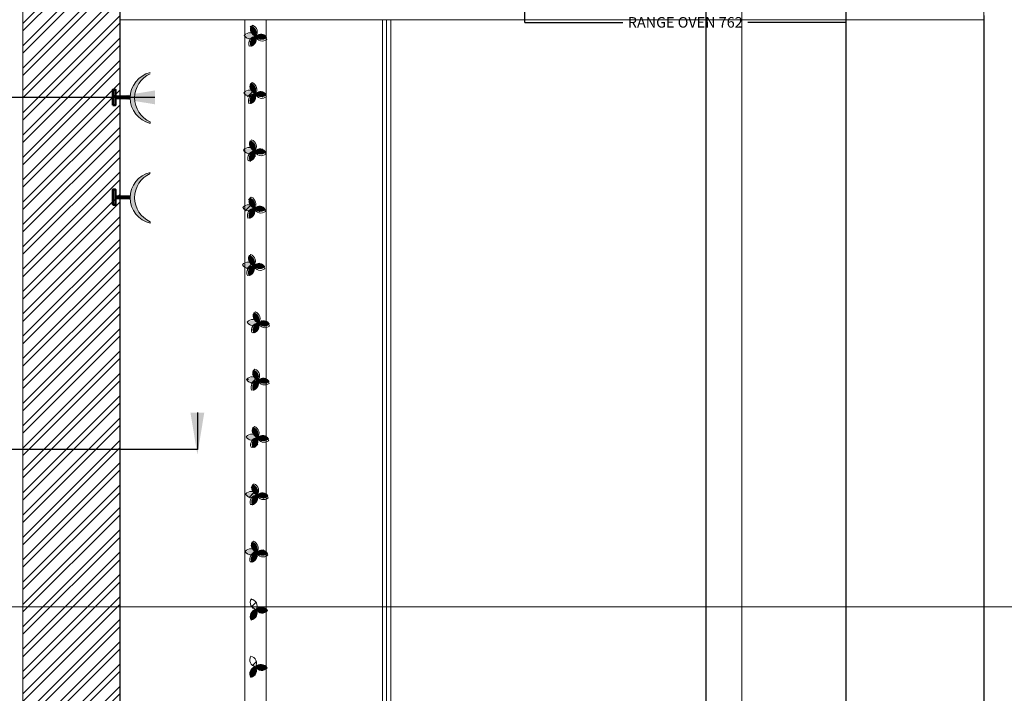
# Model space of a CAD drawing. Units: millimetres. Extents: x 1944 to 29915, y -10550 to 5909.
# Tile 7 of 24: x 6709 to 9044, y 2263 to 3861. Entities that reach past the tile are written whole.
import ezdxf
from ezdxf import colors
from ezdxf.entities.mleader import LeaderData, LeaderLine
from ezdxf.math import Vec2, Vec3

# ---------------------------------------------------------------- set-up
doc = ezdxf.new("R2010")
doc.units = ezdxf.units.MM
doc.header["$MEASUREMENT"] = 0
for name, color, linetype, lineweight in [('A-ANNO-DIMS', 2, 'Continuous', 18), ('A-ANNO-SYMB', 2, 'Continuous', 18), ('A-ANNO-TEXT', 7, 'Continuous', 25), ('A-FLOR-FIXT', 9, 'Continuous', 18), ('A-FLOR-PATT', 252, 'Continuous', 13), ('A-FURN', 8, 'Continuous', 18), ('A-WALL', 7, 'Continuous', 50), ('A-WALL-PATT', 8, 'Continuous', 18)]:
    doc.layers.add(name, color=color, linetype=linetype, lineweight=lineweight)
doc.styles.get("Standard").update_dxf_attribs({"font": 'arial.ttf'})
doc.dimstyles.get("Standard").update_dxf_attribs({"dimtxt": 25, "dimasz": 0.18, "dimexe": 0.18, "dimexo": 0.0625, "dimgap": 0.09, "dimtad": 0, "dimtih": 1, "dimtoh": 1, "dimdec": 0, "dimzin": 0, "dimdsep": 46, "dimtxsty": 'Standard', "dimcen": 0.09, "dimadec": 0, "dimazin": 0, "dimtfac": 1, "dimtdec": 0, "dimtofl": 0, "dimtmove": 0, "dimatfit": 3, "dimfxl": 1, "dimtolj": 1, "dimtzin": 0, "dimarcsym": 0})

# ---------------------------------------------------------------- blocks, each defined once
blk = doc.blocks.new('ORNAMENT-TILE')
for points in [[(27, 25, 0.520567), (15.6, 50, 0.520567)], [(27.4, 25, -0.520567), (0, 23.1, -0.520567)], [(27, 25, -0.520567), (15.6, 0, -0.520567)], [(27, 25, 0.520567), (54.3, 22.2, 0.520567)]]:
    blk.add_lwpolyline(points, format="xyb", close=True)
blk = doc.blocks.new('COAT-HOOK')
blk.add_line((47.6, 3.3), (47.6, 0))
for centre, radius, start, end in [((61.9, 60.2), 61.9, 103.3534, 256.6466), ((73.3, 60.6), 62.7, 114.1736, 245.8264)]:
    blk.add_arc(centre, radius, start, end)
blk = doc.blocks.new('*D38')
at = {"layer": 'A-ANNO-DIMS', "color": 0, "lineweight": -2, "transparency": 16777216}
for p, q in [((7906, 3968.8), (7906, 3854.4)), ((8668, 3968.8), (8668, 3854.4)), ((7906.2, 3854.5), (8138.8, 3854.5)), ((8667.9, 3854.5), (8435.3, 3854.5))]:
    blk.add_line(p, q, dxfattribs=at)
at = {"layer": 'A-ANNO-DIMS', "color": 0, "transparency": 16777216}
for points in [[(7906.2, 3854.6), (7906.2, 3854.5), (7906, 3854.5)], [(8667.9, 3854.6), (8667.9, 3854.5), (8668, 3854.5)]]:
    blk.add_solid(points, dxfattribs=at)
at = {"layer": 'Defpoints', "color": 0, "transparency": 16777216}
for p in [(7906, 3968.8), (8668, 3968.8), (8668, 3854.5)]:
    blk.add_point(p, dxfattribs=at)
at = {"layer": 'A-ANNO-DIMS', "color": 0, "transparency": 16777216, "insert": (8287, 3854.5), "char_height": 25, "attachment_point": 5}
blk.add_mtext('\\A1;RANGE OVEN 762', dxfattribs=at)
blk = doc.blocks.new('*D49')
at = {"layer": 'A-ANNO-DIMS', "color": 0, "lineweight": -2, "transparency": 16777216}
for p, q in [((8335.5, 4760.8), (8335.5, -697.2)), ((6945.9, 4530.8), (6945.9, -697.2)), ((6946.1, -697), (7589.8, -697)), ((8335.3, -697), (7691.6, -697))]:
    blk.add_line(p, q, dxfattribs=at)
at = {"layer": 'A-ANNO-DIMS', "color": 0, "transparency": 16777216}
for points in [[(6946.1, -697), (6946.1, -697.1), (6945.9, -697)], [(8335.3, -697), (8335.3, -697.1), (8335.5, -697)]]:
    blk.add_solid(points, dxfattribs=at)
at = {"layer": 'Defpoints', "color": 0, "transparency": 16777216}
for p in [(8335.5, 4760.8), (6945.9, 4530.8), (8335.5, -697)]:
    blk.add_point(p, dxfattribs=at)
at = {"layer": 'A-ANNO-DIMS', "color": 0, "transparency": 16777216, "insert": (7640.7, -697), "char_height": 25, "attachment_point": 5}
blk.add_mtext('\\A1;1389.5', dxfattribs=at)
blk = doc.blocks.new('*D57')
at = {"layer": 'A-ANNO-DIMS', "color": 0, "lineweight": -2, "transparency": 16777216}
for p, q in [((8995.2, 4760.8), (5803.8, 4760.8)), ((5804, 4760.7), (5804, 2520.7)), ((5804, 255), (5804, 2495)), ((8999.6, 254.8), (5803.8, 254.8))]:
    blk.add_line(p, q, dxfattribs=at)
at = {"layer": 'A-ANNO-DIMS', "color": 0, "transparency": 16777216}
for points in [[(5804, 4760.7), (5804, 4760.7), (5804, 4760.8)], [(5804, 255), (5804, 255), (5804, 254.8)]]:
    blk.add_solid(points, dxfattribs=at)
at = {"layer": 'Defpoints', "color": 0, "transparency": 16777216}
for p in [(8995.2, 4760.8), (5804, 254.8), (8999.6, 254.8)]:
    blk.add_point(p, dxfattribs=at)
at = {"layer": 'A-ANNO-DIMS', "color": 0, "transparency": 16777216, "insert": (5804, 2507.8), "char_height": 25, "attachment_point": 5}
blk.add_mtext('\\A1;4506', dxfattribs=at)
blk = doc.blocks.new('*D59')
at = {"layer": 'A-ANNO-DIMS', "color": 0, "lineweight": -2, "transparency": 16777216}
for p, q in [((8668, 4019.6), (8668, -697.2)), ((8995.2, 3870.8), (8995.2, -697.2)), ((8668.2, -697), (8789.5, -697)), ((8995, -697), (8873.8, -697))]:
    blk.add_line(p, q, dxfattribs=at)
at = {"layer": 'A-ANNO-DIMS', "color": 0, "transparency": 16777216}
for points in [[(8668.2, -697), (8668.2, -697.1), (8668, -697)], [(8995, -697), (8995, -697.1), (8995.2, -697)]]:
    blk.add_solid(points, dxfattribs=at)
at = {"layer": 'Defpoints', "color": 0, "transparency": 16777216}
for p in [(8668, 4019.6), (8995.2, 3870.8), (8995.2, -697)]:
    blk.add_point(p, dxfattribs=at)
at = {"layer": 'A-ANNO-DIMS', "color": 0, "transparency": 16777216, "insert": (8831.6, -697), "char_height": 25, "attachment_point": 5}
blk.add_mtext('\\A1;327.2', dxfattribs=at)

msp = doc.modelspace()

# ---------------------------------------------------------------- hatches: boundary and pattern name
at = {"layer": 'A-ANNO-SYMB'}
h = msp.add_hatch(color=256, dxfattribs=at)
h.dxf.hatch_style = 1
h.paths.add_polyline_path([(7018.308, 3614.925), (7018.308, 3618.232, -0.64725624), (7018.308, 3732.725), (7018.308, 3735.411, 0.79041326)])
h = msp.add_hatch(color=256, dxfattribs=at)
h.dxf.hatch_style = 1
h.paths.add_polyline_path([(6929.507, 3658.332), (6936.053, 3658.332), (6936.053, 3694.562), (6929.507, 3694.562)])
h = msp.add_hatch(color=256, dxfattribs=at)
h.dxf.hatch_style = 1
h.paths.add_polyline_path([(6936.053, 3678.409), (6936.053, 3674.325), (6970.696, 3674.325, -0.01650068), (6970.776, 3678.409)])
h = msp.add_hatch(color=256, dxfattribs=at)
h.dxf.hatch_style = 1
h.paths.add_polyline_path([(7018.308, 3378.048), (7018.308, 3381.355, -0.64725624), (7018.308, 3495.848), (7018.308, 3498.534, 0.79041326)])
h = msp.add_hatch(color=256, dxfattribs=at)
h.dxf.hatch_style = 1
h.paths.add_polyline_path([(6929.507, 3421.455), (6936.053, 3421.455), (6936.053, 3457.684), (6929.507, 3457.684)])
h = msp.add_hatch(color=256, dxfattribs=at)
h.dxf.hatch_style = 1
h.paths.add_polyline_path([(6936.053, 3441.532), (6936.053, 3437.447), (6970.696, 3437.447, -0.01650068), (6970.776, 3441.532)])
at = {"layer": 'A-FLOR-PATT'}
h = msp.add_hatch(color=256, dxfattribs=at)
h.dxf.hatch_style = 1
h.paths.add_polyline_path([(7256.928, 3846.567, -0.52056705), (7268.294, 3821.579, -0.52056705), (7256.928, 3796.591, -0.27363046), (7256.947, 3813.653, -0.26802551), (7241.299, 3819.656, -0.30570263), (7258.281, 3827.577, -0.31162563)])
h = msp.add_hatch(dxfattribs=at)
h.set_pattern_fill('ANSI32', color=256, scale=100)
h.paths.add_polyline_path([(7256.928, 3846.567, 0.31162563), (7258.281, 3827.577, -0.17976414), (7268.452, 3821.853, 0.51458497)])
h = msp.add_hatch(color=256, dxfattribs=at)
h.dxf.hatch_style = 1
h.paths.add_polyline_path([(7256.928, 3846.567, 0.31162563), (7258.281, 3827.577, -0.17976414), (7268.452, 3821.853, 0.51458497)])
h = msp.add_hatch(dxfattribs=at)
h.set_pattern_fill('ANSI32', color=256, scale=100)
h.paths.add_polyline_path([(7268.484, 3821.248, -0.00568537), (7268.294, 3821.579, 0.21614784), (7256.947, 3813.653, 0.21566285)], flags=16)
h.paths.add_polyline_path([(7295.606, 3818.823, -0.51336232), (7268.484, 3821.248, -0.51336232), (7256.928, 3796.591, -0.27363046), (7256.947, 3813.653, -0.26802551), (7241.299, 3819.656, -0.30570263), (7258.281, 3827.577, -0.18072738), (7268.492, 3821.805, -0.51487633)])
h.paths.add_polyline_path([(7268.484, 3821.248, -0.21566285), (7256.947, 3813.653, 0.27363046), (7256.928, 3796.591, 0.51336232)], flags=16)
h = msp.add_hatch(dxfattribs=at)
h.set_pattern_fill('ANSI32', color=256, scale=100)
h.paths.add_polyline_path([(7268.294, 3821.579, -0.17977754), (7258.281, 3827.577, 0.30570263), (7241.299, 3819.656, 0.26802551), (7256.947, 3813.653, -0.21614784)])
h.paths.add_polyline_path([(7268.484, 3821.248, -0.00568537), (7268.294, 3821.579, 0.21614784), (7256.947, 3813.653, 0.21566285)], flags=16)
h.paths.add_polyline_path([(7268.484, 3821.248, -0.21566285), (7256.947, 3813.653, 0.27363046), (7256.928, 3796.591, 0.51336232)], flags=16)
h = msp.add_hatch(color=256, dxfattribs=at)
h.dxf.hatch_style = 1
h.paths.add_polyline_path([(7256.947, 3813.653, 0.27363046), (7256.928, 3796.591, 0.51336232), (7268.484, 3821.248, -0.21566285)])
h = msp.add_hatch(color=256, dxfattribs=at)
h.dxf.hatch_style = 1
h.paths.add_polyline_path([(7268.484, 3821.248, -0.00568537), (7268.294, 3821.579, 0.21614784), (7256.947, 3813.653, 0.21566285)])
h = msp.add_hatch(color=256, dxfattribs=at)
h.dxf.hatch_style = 1
h.paths.add_polyline_path([(7258.281, 3827.577, 0.17977754), (7268.294, 3821.579, 0.00471819), (7268.452, 3821.853, 0.17976414)])
h = msp.add_hatch(color=256, dxfattribs=at)
h.dxf.hatch_style = 1
h.paths.add_polyline_path([(7268.492, 3821.805, -0.00448785), (7268.684, 3821.573, -0.00568537), (7268.484, 3821.248, 0.51336232), (7295.606, 3818.823, 0.51487633)])
h = msp.add_hatch(color=256, dxfattribs=at)
h.dxf.hatch_style = 1
h.paths.add_polyline_path([(7255.798, 3710.561, -0.52056705), (7267.164, 3685.573, -0.52056705), (7255.798, 3660.585, -0.27363046), (7255.818, 3677.648, -0.26802551), (7240.17, 3683.651, -0.30570263), (7257.151, 3691.572, -0.31162563)])
h = msp.add_hatch(dxfattribs=at)
h.set_pattern_fill('ANSI32', color=256, scale=100)
h.paths.add_polyline_path([(7267.354, 3685.243, -0.00568537), (7267.164, 3685.573, 0.21614784), (7255.818, 3677.648, 0.21566285)], flags=16)
h.paths.add_polyline_path([(7294.477, 3682.818, -0.51336232), (7267.354, 3685.243, -0.51336232), (7255.798, 3660.585, -0.27363046), (7255.818, 3677.648, -0.26802551), (7240.17, 3683.651, -0.30570263), (7257.151, 3691.572, -0.18072738), (7267.362, 3685.799, -0.51487633)])
h.paths.add_polyline_path([(7267.354, 3685.243, -0.21566285), (7255.818, 3677.648, 0.27363046), (7255.798, 3660.585, 0.51336232)], flags=16)
h = msp.add_hatch(dxfattribs=at)
h.set_pattern_fill('ANSI32', color=256, scale=100)
h.paths.add_polyline_path([(7267.164, 3685.573, -0.17977754), (7257.151, 3691.572, 0.30570263), (7240.17, 3683.651, 0.26802551), (7255.818, 3677.648, -0.21614784)])
h.paths.add_polyline_path([(7267.354, 3685.243, -0.00568537), (7267.164, 3685.573, 0.21614784), (7255.818, 3677.648, 0.21566285)], flags=16)
h.paths.add_polyline_path([(7267.354, 3685.243, -0.21566285), (7255.818, 3677.648, 0.27363046), (7255.798, 3660.585, 0.51336232)], flags=16)
h = msp.add_hatch(dxfattribs=at)
h.set_pattern_fill('ANSI32', color=256, scale=100)
h.paths.add_polyline_path([(7255.798, 3710.561, 0.31162563), (7257.151, 3691.572, -0.17976414), (7267.322, 3685.847, 0.51458497)])
h = msp.add_hatch(color=256, dxfattribs=at)
h.dxf.hatch_style = 1
h.paths.add_polyline_path([(7255.798, 3710.561, 0.31162563), (7257.151, 3691.572, -0.17976414), (7267.322, 3685.847, 0.51458497)])
h = msp.add_hatch(color=256, dxfattribs=at)
h.dxf.hatch_style = 1
h.paths.add_polyline_path([(7257.151, 3691.572, 0.17977754), (7267.164, 3685.573, 0.00471819), (7267.322, 3685.847, 0.17976414)])
h = msp.add_hatch(color=256, dxfattribs=at)
h.dxf.hatch_style = 1
h.paths.add_polyline_path([(7267.362, 3685.799, -0.00448785), (7267.554, 3685.567, -0.00568537), (7267.354, 3685.243, 0.51336232), (7294.477, 3682.818, 0.51487633)])
h = msp.add_hatch(color=256, dxfattribs=at)
h.dxf.hatch_style = 1
h.paths.add_polyline_path([(7255.818, 3677.648, 0.27363046), (7255.798, 3660.585, 0.51336232), (7267.354, 3685.243, -0.21566285)])
h = msp.add_hatch(color=256, dxfattribs=at)
h.dxf.hatch_style = 1
h.paths.add_polyline_path([(7267.354, 3685.243, -0.00568537), (7267.164, 3685.573, 0.21614784), (7255.818, 3677.648, 0.21566285)])
h = msp.add_hatch(color=256, dxfattribs=at)
h.dxf.hatch_style = 1
h.paths.add_polyline_path([(7254.668, 3574.556, -0.52056705), (7266.034, 3549.568, -0.52056705), (7254.668, 3524.58, -0.27363046), (7254.688, 3541.642, -0.26802551), (7239.04, 3547.645, -0.30570263), (7256.021, 3555.566, -0.31162563)])
h = msp.add_hatch(dxfattribs=at)
h.set_pattern_fill('ANSI32', color=256, scale=100)
h.paths.add_polyline_path([(7254.668, 3574.556, 0.31162563), (7256.021, 3555.566, -0.17976414), (7266.192, 3549.842, 0.51458497)])
h = msp.add_hatch(color=256, dxfattribs=at)
h.dxf.hatch_style = 1
h.paths.add_polyline_path([(7254.668, 3574.556, 0.31162563), (7256.021, 3555.566, -0.17976414), (7266.192, 3549.842, 0.51458497)])
h = msp.add_hatch(dxfattribs=at)
h.set_pattern_fill('ANSI32', color=256, scale=100)
h.paths.add_polyline_path([(7266.224, 3549.238, -0.00568537), (7266.034, 3549.568, 0.21614784), (7254.688, 3541.642, 0.21566285)], flags=16)
h.paths.add_polyline_path([(7293.347, 3546.812, -0.51336232), (7266.224, 3549.238, -0.51336232), (7254.668, 3524.58, -0.27363046), (7254.688, 3541.642, -0.26802551), (7239.04, 3547.645, -0.30570263), (7256.021, 3555.566, -0.18072738), (7266.233, 3549.794, -0.51487633)])
h.paths.add_polyline_path([(7266.224, 3549.238, -0.21566285), (7254.688, 3541.642, 0.27363046), (7254.668, 3524.58, 0.51336232)], flags=16)
h = msp.add_hatch(dxfattribs=at)
h.set_pattern_fill('ANSI32', color=256, scale=100)
h.paths.add_polyline_path([(7266.034, 3549.568, -0.17977754), (7256.021, 3555.566, 0.30570263), (7239.04, 3547.645, 0.26802551), (7254.688, 3541.642, -0.21614784)])
h.paths.add_polyline_path([(7266.224, 3549.238, -0.00568537), (7266.034, 3549.568, 0.21614784), (7254.688, 3541.642, 0.21566285)], flags=16)
h.paths.add_polyline_path([(7266.224, 3549.238, -0.21566285), (7254.688, 3541.642, 0.27363046), (7254.668, 3524.58, 0.51336232)], flags=16)
h = msp.add_hatch(color=256, dxfattribs=at)
h.dxf.hatch_style = 1
h.paths.add_polyline_path([(7254.688, 3541.642, 0.27363046), (7254.668, 3524.58, 0.51336232), (7266.224, 3549.238, -0.21566285)])
h = msp.add_hatch(color=256, dxfattribs=at)
h.dxf.hatch_style = 1
h.paths.add_polyline_path([(7266.224, 3549.238, -0.00568537), (7266.034, 3549.568, 0.21614784), (7254.688, 3541.642, 0.21566285)])
h = msp.add_hatch(color=256, dxfattribs=at)
h.dxf.hatch_style = 1
h.paths.add_polyline_path([(7256.021, 3555.566, 0.17977754), (7266.034, 3549.568, 0.00471819), (7266.192, 3549.842, 0.17976414)])
h = msp.add_hatch(color=256, dxfattribs=at)
h.dxf.hatch_style = 1
h.paths.add_polyline_path([(7266.233, 3549.794, -0.00448785), (7266.424, 3549.562, -0.00568537), (7266.224, 3549.238, 0.51336232), (7293.347, 3546.812, 0.51487633)])
h = msp.add_hatch(color=256, dxfattribs=at)
h.dxf.hatch_style = 1
h.paths.add_polyline_path([(7253.539, 3438.55, -0.52056705), (7264.904, 3413.563, -0.52056705), (7253.539, 3388.575, -0.27363046), (7253.558, 3405.637, -0.26802551), (7237.91, 3411.64, -0.30570263), (7254.892, 3419.561, -0.31162563)])
h = msp.add_hatch(dxfattribs=at)
h.set_pattern_fill('ANSI32', color=256, scale=100)
h.paths.add_polyline_path([(7253.539, 3438.55, 0.31162563), (7254.892, 3419.561, -0.17976414), (7265.063, 3413.836, 0.51458497)])
h = msp.add_hatch(color=256, dxfattribs=at)
h.dxf.hatch_style = 1
h.paths.add_polyline_path([(7253.539, 3438.55, 0.31162563), (7254.892, 3419.561, -0.17976414), (7265.063, 3413.836, 0.51458497)])
h = msp.add_hatch(dxfattribs=at)
h.set_pattern_fill('ANSI32', color=256, scale=100)
h.paths.add_polyline_path([(7265.094, 3413.232, -0.00568537), (7264.904, 3413.563, 0.21614784), (7253.558, 3405.637, 0.21566285)], flags=16)
h.paths.add_polyline_path([(7292.217, 3410.807, -0.51336232), (7265.094, 3413.232, -0.51336232), (7253.539, 3388.575, -0.27363046), (7253.558, 3405.637, -0.26802551), (7237.91, 3411.64, -0.30570263), (7254.892, 3419.561, -0.18072738), (7265.103, 3413.789, -0.51487633)])
h.paths.add_polyline_path([(7265.094, 3413.232, -0.21566285), (7253.558, 3405.637, 0.27363046), (7253.539, 3388.575, 0.51336232)], flags=16)
h = msp.add_hatch(dxfattribs=at)
h.set_pattern_fill('ANSI32', color=256, scale=100)
h.paths.add_polyline_path([(7264.904, 3413.563, -0.17977754), (7254.892, 3419.561, 0.30570263), (7237.91, 3411.64, 0.26802551), (7253.558, 3405.637, -0.21614784)])
h.paths.add_polyline_path([(7265.094, 3413.232, -0.00568537), (7264.904, 3413.563, 0.21614784), (7253.558, 3405.637, 0.21566285)], flags=16)
h.paths.add_polyline_path([(7265.094, 3413.232, -0.21566285), (7253.558, 3405.637, 0.27363046), (7253.539, 3388.575, 0.51336232)], flags=16)
h = msp.add_hatch(color=256, dxfattribs=at)
h.dxf.hatch_style = 1
h.paths.add_polyline_path([(7253.558, 3405.637, 0.27363046), (7253.539, 3388.575, 0.51336232), (7265.094, 3413.232, -0.21566285)])
h = msp.add_hatch(color=256, dxfattribs=at)
h.dxf.hatch_style = 1
h.paths.add_polyline_path([(7265.094, 3413.232, -0.00568537), (7264.904, 3413.563, 0.21614784), (7253.558, 3405.637, 0.21566285)])
h = msp.add_hatch(color=256, dxfattribs=at)
h.dxf.hatch_style = 1
h.paths.add_polyline_path([(7254.892, 3419.561, 0.17977754), (7264.904, 3413.563, 0.00471819), (7265.063, 3413.836, 0.17976414)])
h = msp.add_hatch(color=256, dxfattribs=at)
h.dxf.hatch_style = 1
h.paths.add_polyline_path([(7265.103, 3413.789, -0.00448785), (7265.294, 3413.557, -0.00568537), (7265.094, 3413.232, 0.51336232), (7292.217, 3410.807, 0.51487633)])
h = msp.add_hatch(color=256, dxfattribs=at)
h.dxf.hatch_style = 1
h.paths.add_polyline_path([(7252.409, 3302.545, -0.52056705), (7263.775, 3277.557, -0.52056705), (7252.409, 3252.569, -0.27363046), (7252.428, 3269.631, -0.26802551), (7236.78, 3275.635, -0.30570263), (7253.762, 3283.556, -0.31162563)])
h = msp.add_hatch(dxfattribs=at)
h.set_pattern_fill('ANSI32', color=256, scale=100)
h.paths.add_polyline_path([(7252.409, 3302.545, 0.31162563), (7253.762, 3283.556, -0.17976414), (7263.933, 3277.831, 0.51458497)])
h = msp.add_hatch(color=256, dxfattribs=at)
h.dxf.hatch_style = 1
h.paths.add_polyline_path([(7252.409, 3302.545, 0.31162563), (7253.762, 3283.556, -0.17976414), (7263.933, 3277.831, 0.51458497)])
h = msp.add_hatch(dxfattribs=at)
h.set_pattern_fill('ANSI32', color=256, scale=100)
h.paths.add_polyline_path([(7263.965, 3277.227, -0.00568537), (7263.775, 3277.557, 0.21614784), (7252.428, 3269.631, 0.21566285)], flags=16)
h.paths.add_polyline_path([(7291.087, 3274.801, -0.51336232), (7263.965, 3277.227, -0.51336232), (7252.409, 3252.569, -0.27363046), (7252.428, 3269.631, -0.26802551), (7236.78, 3275.635, -0.30570263), (7253.762, 3283.556, -0.18072738), (7263.973, 3277.783, -0.51487633)])
h.paths.add_polyline_path([(7263.965, 3277.227, -0.21566285), (7252.428, 3269.631, 0.27363046), (7252.409, 3252.569, 0.51336232)], flags=16)
h = msp.add_hatch(dxfattribs=at)
h.set_pattern_fill('ANSI32', color=256, scale=100)
h.paths.add_polyline_path([(7263.775, 3277.557, -0.17977754), (7253.762, 3283.556, 0.30570263), (7236.78, 3275.635, 0.26802551), (7252.428, 3269.631, -0.21614784)])
h.paths.add_polyline_path([(7263.965, 3277.227, -0.00568537), (7263.775, 3277.557, 0.21614784), (7252.428, 3269.631, 0.21566285)], flags=16)
h.paths.add_polyline_path([(7263.965, 3277.227, -0.21566285), (7252.428, 3269.631, 0.27363046), (7252.409, 3252.569, 0.51336232)], flags=16)
h = msp.add_hatch(color=256, dxfattribs=at)
h.dxf.hatch_style = 1
h.paths.add_polyline_path([(7252.428, 3269.631, 0.27363046), (7252.409, 3252.569, 0.51336232), (7263.965, 3277.227, -0.21566285)])
h = msp.add_hatch(color=256, dxfattribs=at)
h.dxf.hatch_style = 1
h.paths.add_polyline_path([(7263.965, 3277.227, -0.00568537), (7263.775, 3277.557, 0.21614784), (7252.428, 3269.631, 0.21566285)])
h = msp.add_hatch(color=256, dxfattribs=at)
h.dxf.hatch_style = 1
h.paths.add_polyline_path([(7253.762, 3283.556, 0.17977754), (7263.775, 3277.557, 0.00471819), (7263.933, 3277.831, 0.17976414)])
h = msp.add_hatch(color=256, dxfattribs=at)
h.dxf.hatch_style = 1
h.paths.add_polyline_path([(7263.973, 3277.783, -0.00448785), (7264.164, 3277.551, -0.00568537), (7263.965, 3277.227, 0.51336232), (7291.087, 3274.801, 0.51487633)])
h = msp.add_hatch(color=256, dxfattribs=at)
h.dxf.hatch_style = 1
h.paths.add_polyline_path([(7263.491, 3166.54, -0.52056705), (7274.857, 3141.552, -0.52056705), (7263.491, 3116.564, -0.27363046), (7263.51, 3133.626, -0.26802551), (7247.862, 3139.629, -0.30570263), (7264.844, 3147.55, -0.31162563)])
h = msp.add_hatch(dxfattribs=at)
h.set_pattern_fill('ANSI32', color=256, scale=100)
h.paths.add_polyline_path([(7263.491, 3166.54, 0.31162563), (7264.844, 3147.55, -0.17976414), (7275.015, 3141.826, 0.51458497)])
h = msp.add_hatch(color=256, dxfattribs=at)
h.dxf.hatch_style = 1
h.paths.add_polyline_path([(7263.491, 3166.54, 0.31162563), (7264.844, 3147.55, -0.17976414), (7275.015, 3141.826, 0.51458497)])
h = msp.add_hatch(dxfattribs=at)
h.set_pattern_fill('ANSI32', color=256, scale=100)
h.paths.add_polyline_path([(7275.047, 3141.221, -0.00568537), (7274.857, 3141.552, 0.21614784), (7263.51, 3133.626, 0.21566285)], flags=16)
h.paths.add_polyline_path([(7302.17, 3138.796, -0.51336232), (7275.047, 3141.221, -0.51336232), (7263.491, 3116.564, -0.27363046), (7263.51, 3133.626, -0.26802551), (7247.862, 3139.629, -0.30570263), (7264.844, 3147.55, -0.18072738), (7275.055, 3141.778, -0.51487633)])
h.paths.add_polyline_path([(7275.047, 3141.221, -0.21566285), (7263.51, 3133.626, 0.27363046), (7263.491, 3116.564, 0.51336232)], flags=16)
h = msp.add_hatch(dxfattribs=at)
h.set_pattern_fill('ANSI32', color=256, scale=100)
h.paths.add_polyline_path([(7274.857, 3141.552, -0.17977754), (7264.844, 3147.55, 0.30570263), (7247.862, 3139.629, 0.26802551), (7263.51, 3133.626, -0.21614784)])
h.paths.add_polyline_path([(7275.047, 3141.221, -0.00568537), (7274.857, 3141.552, 0.21614784), (7263.51, 3133.626, 0.21566285)], flags=16)
h.paths.add_polyline_path([(7275.047, 3141.221, -0.21566285), (7263.51, 3133.626, 0.27363046), (7263.491, 3116.564, 0.51336232)], flags=16)
h = msp.add_hatch(color=256, dxfattribs=at)
h.dxf.hatch_style = 1
h.paths.add_polyline_path([(7263.51, 3133.626, 0.27363046), (7263.491, 3116.564, 0.51336232), (7275.047, 3141.221, -0.21566285)])
h = msp.add_hatch(color=256, dxfattribs=at)
h.dxf.hatch_style = 1
h.paths.add_polyline_path([(7275.047, 3141.221, -0.00568537), (7274.857, 3141.552, 0.21614784), (7263.51, 3133.626, 0.21566285)])
h = msp.add_hatch(color=256, dxfattribs=at)
h.dxf.hatch_style = 1
h.paths.add_polyline_path([(7264.844, 3147.55, 0.17977754), (7274.857, 3141.552, 0.00471819), (7275.015, 3141.826, 0.17976414)])
h = msp.add_hatch(color=256, dxfattribs=at)
h.dxf.hatch_style = 1
h.paths.add_polyline_path([(7275.055, 3141.778, -0.00448785), (7275.247, 3141.546, -0.00568537), (7275.047, 3141.221, 0.51336232), (7302.17, 3138.796, 0.51487633)])
h = msp.add_hatch(color=256, dxfattribs=at)
h.dxf.hatch_style = 1
h.paths.add_polyline_path([(7262.361, 3030.534, -0.52056705), (7273.727, 3005.546, -0.52056705), (7262.361, 2980.558, -0.27363046), (7262.381, 2997.621, -0.26802551), (7246.733, 3003.624, -0.30570263), (7263.714, 3011.545, -0.31162563)])
h = msp.add_hatch(dxfattribs=at)
h.set_pattern_fill('ANSI32', color=256, scale=100)
h.paths.add_polyline_path([(7262.361, 3030.534, 0.31162563), (7263.714, 3011.545, -0.17976414), (7273.885, 3005.82, 0.51458497)])
h = msp.add_hatch(color=256, dxfattribs=at)
h.dxf.hatch_style = 1
h.paths.add_polyline_path([(7262.361, 3030.534, 0.31162563), (7263.714, 3011.545, -0.17976414), (7273.885, 3005.82, 0.51458497)])
h = msp.add_hatch(dxfattribs=at)
h.set_pattern_fill('ANSI32', color=256, scale=100)
h.paths.add_polyline_path([(7273.917, 3005.216, -0.00568537), (7273.727, 3005.546, 0.21614784), (7262.381, 2997.621, 0.21566285)], flags=16)
h.paths.add_polyline_path([(7301.04, 3002.791, -0.51336232), (7273.917, 3005.216, -0.51336232), (7262.361, 2980.558, -0.27363046), (7262.381, 2997.621, -0.26802551), (7246.733, 3003.624, -0.30570263), (7263.714, 3011.545, -0.18072738), (7273.926, 3005.772, -0.51487633)])
h.paths.add_polyline_path([(7273.917, 3005.216, -0.21566285), (7262.381, 2997.621, 0.27363046), (7262.361, 2980.558, 0.51336232)], flags=16)
h = msp.add_hatch(dxfattribs=at)
h.set_pattern_fill('ANSI32', color=256, scale=100)
h.paths.add_polyline_path([(7273.727, 3005.546, -0.17977754), (7263.714, 3011.545, 0.30570263), (7246.733, 3003.624, 0.26802551), (7262.381, 2997.621, -0.21614784)])
h.paths.add_polyline_path([(7273.917, 3005.216, -0.00568537), (7273.727, 3005.546, 0.21614784), (7262.381, 2997.621, 0.21566285)], flags=16)
h.paths.add_polyline_path([(7273.917, 3005.216, -0.21566285), (7262.381, 2997.621, 0.27363046), (7262.361, 2980.558, 0.51336232)], flags=16)
h = msp.add_hatch(color=256, dxfattribs=at)
h.dxf.hatch_style = 1
h.paths.add_polyline_path([(7262.381, 2997.621, 0.27363046), (7262.361, 2980.558, 0.51336232), (7273.917, 3005.216, -0.21566285)])
h = msp.add_hatch(color=256, dxfattribs=at)
h.dxf.hatch_style = 1
h.paths.add_polyline_path([(7273.917, 3005.216, -0.00568537), (7273.727, 3005.546, 0.21614784), (7262.381, 2997.621, 0.21566285)])
h = msp.add_hatch(color=256, dxfattribs=at)
h.dxf.hatch_style = 1
h.paths.add_polyline_path([(7263.714, 3011.545, 0.17977754), (7273.727, 3005.546, 0.00471819), (7273.885, 3005.82, 0.17976414)])
h = msp.add_hatch(color=256, dxfattribs=at)
h.dxf.hatch_style = 1
h.paths.add_polyline_path([(7273.926, 3005.772, -0.00448785), (7274.117, 3005.54, -0.00568537), (7273.917, 3005.216, 0.51336232), (7301.04, 3002.791, 0.51487633)])
h = msp.add_hatch(color=256, dxfattribs=at)
h.dxf.hatch_style = 1
h.paths.add_polyline_path([(7261.232, 2894.529, -0.52056705), (7272.597, 2869.541, -0.52056705), (7261.232, 2844.553, -0.27363046), (7261.251, 2861.615, -0.26802551), (7245.603, 2867.618, -0.30570263), (7262.584, 2875.539, -0.31162563)])
h = msp.add_hatch(dxfattribs=at)
h.set_pattern_fill('ANSI32', color=256, scale=100)
h.paths.add_polyline_path([(7272.787, 2869.211, -0.00568537), (7272.597, 2869.541, 0.21614784), (7261.251, 2861.615, 0.21566285)], flags=16)
h.paths.add_polyline_path([(7299.91, 2866.785, -0.51336232), (7272.787, 2869.211, -0.51336232), (7261.232, 2844.553, -0.27363046), (7261.251, 2861.615, -0.26802551), (7245.603, 2867.618, -0.30570263), (7262.584, 2875.539, -0.18072738), (7272.796, 2869.767, -0.51487633)])
h.paths.add_polyline_path([(7272.787, 2869.211, -0.21566285), (7261.251, 2861.615, 0.27363046), (7261.232, 2844.553, 0.51336232)], flags=16)
h = msp.add_hatch(dxfattribs=at)
h.set_pattern_fill('ANSI32', color=256, scale=100)
h.paths.add_polyline_path([(7272.597, 2869.541, -0.17977754), (7262.584, 2875.539, 0.30570263), (7245.603, 2867.618, 0.26802551), (7261.251, 2861.615, -0.21614784)])
h.paths.add_polyline_path([(7272.787, 2869.211, -0.00568537), (7272.597, 2869.541, 0.21614784), (7261.251, 2861.615, 0.21566285)], flags=16)
h.paths.add_polyline_path([(7272.787, 2869.211, -0.21566285), (7261.251, 2861.615, 0.27363046), (7261.232, 2844.553, 0.51336232)], flags=16)
h = msp.add_hatch(dxfattribs=at)
h.set_pattern_fill('ANSI32', color=256, scale=100)
h.paths.add_polyline_path([(7261.232, 2894.529, 0.31162563), (7262.584, 2875.539, -0.17976414), (7272.755, 2869.815, 0.51458497)])
h = msp.add_hatch(color=256, dxfattribs=at)
h.dxf.hatch_style = 1
h.paths.add_polyline_path([(7261.232, 2894.529, 0.31162563), (7262.584, 2875.539, -0.17976414), (7272.755, 2869.815, 0.51458497)])
h = msp.add_hatch(color=256, dxfattribs=at)
h.dxf.hatch_style = 1
h.paths.add_polyline_path([(7262.584, 2875.539, 0.17977754), (7272.597, 2869.541, 0.00471819), (7272.755, 2869.815, 0.17976414)])
h = msp.add_hatch(color=256, dxfattribs=at)
h.dxf.hatch_style = 1
h.paths.add_polyline_path([(7272.796, 2869.767, -0.00448785), (7272.987, 2869.535, -0.00568537), (7272.787, 2869.211, 0.51336232), (7299.91, 2866.785, 0.51487633)])
h = msp.add_hatch(color=256, dxfattribs=at)
h.dxf.hatch_style = 1
h.paths.add_polyline_path([(7261.251, 2861.615, 0.27363046), (7261.232, 2844.553, 0.51336232), (7272.787, 2869.211, -0.21566285)])
h = msp.add_hatch(color=256, dxfattribs=at)
h.dxf.hatch_style = 1
h.paths.add_polyline_path([(7272.787, 2869.211, -0.00568537), (7272.597, 2869.541, 0.21614784), (7261.251, 2861.615, 0.21566285)])
h = msp.add_hatch(color=256, dxfattribs=at)
h.dxf.hatch_style = 1
h.paths.add_polyline_path([(7260.102, 2758.523, -0.52056705), (7271.467, 2733.536, -0.52056705), (7260.102, 2708.548, -0.27363046), (7260.121, 2725.61, -0.26802551), (7244.473, 2731.613, -0.30570263), (7261.455, 2739.534, -0.31162563)])
h = msp.add_hatch(dxfattribs=at)
h.set_pattern_fill('ANSI32', color=256, scale=100)
h.paths.add_polyline_path([(7260.102, 2758.523, 0.31162563), (7261.455, 2739.534, -0.17976414), (7271.626, 2733.809, 0.51458497)])
h = msp.add_hatch(color=256, dxfattribs=at)
h.dxf.hatch_style = 1
h.paths.add_polyline_path([(7260.102, 2758.523, 0.31162563), (7261.455, 2739.534, -0.17976414), (7271.626, 2733.809, 0.51458497)])
h = msp.add_hatch(dxfattribs=at)
h.set_pattern_fill('ANSI32', color=256, scale=100)
h.paths.add_polyline_path([(7271.657, 2733.205, -0.00568537), (7271.467, 2733.536, 0.21614784), (7260.121, 2725.61, 0.21566285)], flags=16)
h.paths.add_polyline_path([(7298.78, 2730.78, -0.51336232), (7271.657, 2733.205, -0.51336232), (7260.102, 2708.548, -0.27363046), (7260.121, 2725.61, -0.26802551), (7244.473, 2731.613, -0.30570263), (7261.455, 2739.534, -0.18072738), (7271.666, 2733.762, -0.51487633)])
h.paths.add_polyline_path([(7271.657, 2733.205, -0.21566285), (7260.121, 2725.61, 0.27363046), (7260.102, 2708.548, 0.51336232)], flags=16)
h = msp.add_hatch(dxfattribs=at)
h.set_pattern_fill('ANSI32', color=256, scale=100)
h.paths.add_polyline_path([(7271.467, 2733.536, -0.17977754), (7261.455, 2739.534, 0.30570263), (7244.473, 2731.613, 0.26802551), (7260.121, 2725.61, -0.21614784)])
h.paths.add_polyline_path([(7271.657, 2733.205, -0.00568537), (7271.467, 2733.536, 0.21614784), (7260.121, 2725.61, 0.21566285)], flags=16)
h.paths.add_polyline_path([(7271.657, 2733.205, -0.21566285), (7260.121, 2725.61, 0.27363046), (7260.102, 2708.548, 0.51336232)], flags=16)
h = msp.add_hatch(color=256, dxfattribs=at)
h.dxf.hatch_style = 1
h.paths.add_polyline_path([(7260.121, 2725.61, 0.27363046), (7260.102, 2708.548, 0.51336232), (7271.657, 2733.205, -0.21566285)])
h = msp.add_hatch(color=256, dxfattribs=at)
h.dxf.hatch_style = 1
h.paths.add_polyline_path([(7271.657, 2733.205, -0.00568537), (7271.467, 2733.536, 0.21614784), (7260.121, 2725.61, 0.21566285)])
h = msp.add_hatch(color=256, dxfattribs=at)
h.dxf.hatch_style = 1
h.paths.add_polyline_path([(7261.455, 2739.534, 0.17977754), (7271.467, 2733.536, 0.00471819), (7271.626, 2733.809, 0.17976414)])
h = msp.add_hatch(color=256, dxfattribs=at)
h.dxf.hatch_style = 1
h.paths.add_polyline_path([(7271.666, 2733.762, -0.00448785), (7271.857, 2733.53, -0.00568537), (7271.657, 2733.205, 0.51336232), (7298.78, 2730.78, 0.51487633)])
h = msp.add_hatch(color=256, dxfattribs=at)
h.dxf.hatch_style = 1
h.paths.add_polyline_path([(7258.972, 2622.518, -0.52056705), (7270.338, 2597.53, -0.52056705), (7258.972, 2572.542, -0.27363046), (7258.991, 2589.604, -0.26802551), (7243.343, 2595.608, -0.30570263), (7260.325, 2603.529, -0.31162563)])
h = msp.add_hatch(dxfattribs=at)
h.set_pattern_fill('ANSI32', color=256, scale=100)
h.paths.add_polyline_path([(7258.972, 2622.518, 0.31162563), (7260.325, 2603.529, -0.17976414), (7270.496, 2597.804, 0.51458497)])
h = msp.add_hatch(color=256, dxfattribs=at)
h.dxf.hatch_style = 1
h.paths.add_polyline_path([(7258.972, 2622.518, 0.31162563), (7260.325, 2603.529, -0.17976414), (7270.496, 2597.804, 0.51458497)])
h = msp.add_hatch(dxfattribs=at)
h.set_pattern_fill('ANSI32', color=256, scale=100)
h.paths.add_polyline_path([(7270.528, 2597.2, -0.00568537), (7270.338, 2597.53, 0.21614784), (7258.991, 2589.604, 0.21566285)], flags=16)
h.paths.add_polyline_path([(7297.65, 2594.774, -0.51336232), (7270.528, 2597.2, -0.51336232), (7258.972, 2572.542, -0.27363046), (7258.991, 2589.604, -0.26802551), (7243.343, 2595.608, -0.30570263), (7260.325, 2603.529, -0.18072738), (7270.536, 2597.756, -0.51487633)])
h.paths.add_polyline_path([(7270.528, 2597.2, -0.21566285), (7258.991, 2589.604, 0.27363046), (7258.972, 2572.542, 0.51336232)], flags=16)
h = msp.add_hatch(dxfattribs=at)
h.set_pattern_fill('ANSI32', color=256, scale=100)
h.paths.add_polyline_path([(7270.338, 2597.53, -0.17977754), (7260.325, 2603.529, 0.30570263), (7243.343, 2595.608, 0.26802551), (7258.991, 2589.604, -0.21614784)])
h.paths.add_polyline_path([(7270.528, 2597.2, -0.00568537), (7270.338, 2597.53, 0.21614784), (7258.991, 2589.604, 0.21566285)], flags=16)
h.paths.add_polyline_path([(7270.528, 2597.2, -0.21566285), (7258.991, 2589.604, 0.27363046), (7258.972, 2572.542, 0.51336232)], flags=16)
h = msp.add_hatch(color=256, dxfattribs=at)
h.dxf.hatch_style = 1
h.paths.add_polyline_path([(7258.991, 2589.604, 0.27363046), (7258.972, 2572.542, 0.51336232), (7270.528, 2597.2, -0.21566285)])
h = msp.add_hatch(color=256, dxfattribs=at)
h.dxf.hatch_style = 1
h.paths.add_polyline_path([(7270.528, 2597.2, -0.00568537), (7270.338, 2597.53, 0.21614784), (7258.991, 2589.604, 0.21566285)])
h = msp.add_hatch(color=256, dxfattribs=at)
h.dxf.hatch_style = 1
h.paths.add_polyline_path([(7260.325, 2603.529, 0.17977754), (7270.338, 2597.53, 0.00471819), (7270.496, 2597.804, 0.17976414)])
h = msp.add_hatch(color=256, dxfattribs=at)
h.dxf.hatch_style = 1
h.paths.add_polyline_path([(7270.536, 2597.756, -0.00448785), (7270.728, 2597.524, -0.00568537), (7270.528, 2597.2, 0.51336232), (7297.65, 2594.774, 0.51487633)])
h = msp.add_hatch(dxfattribs=at)
h.set_pattern_fill('ANSI32', color=256, scale=100)
h.paths.add_polyline_path([(7257.842, 2486.513, 0.31162563), (7259.195, 2467.523, -0.17976414), (7269.366, 2461.799, 0.51458497)])
h = msp.add_hatch(color=256, dxfattribs=at)
h.dxf.hatch_style = 1
h.paths.add_polyline_path([(7257.861, 2453.599, 0.27363046), (7257.842, 2436.537, 0.51336232), (7269.398, 2461.194, -0.21566285)])
h = msp.add_hatch(color=256, dxfattribs=at)
h.dxf.hatch_style = 1
h.paths.add_polyline_path([(7269.398, 2461.194, -0.00568537), (7269.208, 2461.525, 0.21614784), (7257.861, 2453.599, 0.21566285)])
h = msp.add_hatch(color=256, dxfattribs=at)
h.dxf.hatch_style = 1
h.paths.add_polyline_path([(7259.195, 2467.523, 0.17977754), (7269.208, 2461.525, 0.00471819), (7269.366, 2461.799, 0.17976414)])
h = msp.add_hatch(color=256, dxfattribs=at)
h.dxf.hatch_style = 1
h.paths.add_polyline_path([(7269.406, 2461.751, -0.00448785), (7269.598, 2461.519, -0.00568537), (7269.398, 2461.194, 0.51336232), (7296.521, 2458.769, 0.51487633)])
h = msp.add_hatch(dxfattribs=at)
h.set_pattern_fill('ANSI32', color=256, scale=100)
h.paths.add_polyline_path([(7256.712, 2350.507, 0.31162563), (7258.065, 2331.518, -0.17976414), (7268.236, 2325.793, 0.51458497)])
h = msp.add_hatch(color=256, dxfattribs=at)
h.dxf.hatch_style = 1
h.paths.add_polyline_path([(7256.732, 2317.594, 0.27363046), (7256.712, 2300.531, 0.51336232), (7268.268, 2325.189, -0.21566285)])
h = msp.add_hatch(color=256, dxfattribs=at)
h.dxf.hatch_style = 1
h.paths.add_polyline_path([(7268.268, 2325.189, -0.00568537), (7268.078, 2325.519, 0.21614784), (7256.732, 2317.594, 0.21566285)])
h = msp.add_hatch(color=256, dxfattribs=at)
h.dxf.hatch_style = 1
h.paths.add_polyline_path([(7258.065, 2331.518, 0.17977754), (7268.078, 2325.519, 0.00471819), (7268.236, 2325.793, 0.17976414)])
h = msp.add_hatch(color=256, dxfattribs=at)
h.dxf.hatch_style = 1
h.paths.add_polyline_path([(7268.277, 2325.745, -0.00448785), (7268.468, 2325.513, -0.00568537), (7268.268, 2325.189, 0.51336232), (7295.391, 2322.764, 0.51487633)])
at = {"layer": 'A-WALL-PATT'}
h = msp.add_hatch(dxfattribs=at)
h.set_pattern_fill('ANSI32', color=256, scale=100)
h.paths.add_polyline_path([(6945.942, 4530.837), (6715.942, 4530.837), (6715.942, 490.837), (6945.942, 490.837)])

# ---------------------------------------------------------------- linework, layer by layer
at = {"layer": 'A-ANNO-SYMB'}
for p, q in [((8420.942, -176.269), (8420.942, 5412.489)), ((6293.436, 2468.085), (10483.966, 2468.085))]:
    msp.add_line(p, q, dxfattribs=at)
at = {"layer": 'A-FLOR-FIXT'}
for p, q in [((8995.217, 4760.837), (8995.217, 3860.837)), ((8995.217, 3860.837), (6945.942, 3860.837)), ((7242.862, 1207.97), (7242.862, 3860.837)), ((7292.862, 1207.97), (7292.862, 3860.837)), ((7568.787, 3860.837), (7568.787, 260.837)), ((7578.787, 3860.837), (7578.787, 260.837)), ((7578.787, 3860.837), (7578.787, 260.837)), ((7588.787, 3860.837), (7588.787, 260.837))]:
    msp.add_line(p, q, dxfattribs=at)
for points in [[(8995.217, 30.837), (6715.942, 30.837), (6715.942, 4990.837), (8315.477, 4990.837)], [(9000.245, 260.837), (6945.942, 260.837), (6945.942, 4760.837), (8315.477, 4760.837)]]:
    msp.add_lwpolyline(points, dxfattribs=at)
for points in [[(7269.208, 2461.525, 0.52056705), (7257.842, 2486.513, 0.52056705)], [(7269.208, 2461.525, -0.52056705), (7257.842, 2436.537, -0.52056705)], [(7269.208, 2461.525, 0.52056705), (7296.521, 2458.769, 0.52056705)], [(7268.078, 2325.519, 0.52056705), (7256.712, 2350.507, 0.52056705)], [(7268.078, 2325.519, -0.52056705), (7256.712, 2300.531, -0.52056705)], [(7268.078, 2325.519, 0.52056705), (7295.391, 2322.764, 0.52056705)]]:
    msp.add_lwpolyline(points, format="xyb", close=True, dxfattribs=at)
at = {"layer": 'A-WALL'}
for p, q in [((6970.759, 3678.409), (6936.053, 3678.409)), ((6970.759, 3674.325), (6936.053, 3674.325)), ((6970.759, 3441.532), (6936.053, 3441.532)), ((6970.759, 3437.447), (6936.053, 3437.447))]:
    msp.add_line(p, q, dxfattribs=at)
for points in [[(6929.507, 3658.332), (6929.507, 3694.562), (6936.053, 3694.562), (6936.053, 3658.332)], [(6929.507, 3421.455), (6929.507, 3457.684), (6936.053, 3457.684), (6936.053, 3421.455)]]:
    msp.add_lwpolyline(points, close=True, dxfattribs=at)

# ---------------------------------------------------------------- block references
at = {"layer": 'A-FLOR-PATT'}
for p, rotation in [((7237.745, 3800.744), 350.9047073759592), ((7236.615, 3664.738), 350.9047073759626), ((7235.485, 3528.733), 350.904707375963), ((7234.355, 3392.727), 350.9047073759607), ((7233.226, 3256.722), 350.9047073759626), ((7244.308, 3120.717), 350.9047073759577), ((7243.178, 2984.711), 350.9047073759626), ((7242.048, 2848.706), 350.9047073759635), ((7240.918, 2712.7), 350.9047073759597), ((7239.789, 2576.695), 350.9047073759626)]:
    msp.add_blockref('ORNAMENT-TILE', p, dxfattribs=dict(at, rotation=rotation))
at = {"layer": 'A-FURN'}
msp.add_blockref('COAT-HOOK', (6970.691, 3614.925), dxfattribs=at)
at = {"layer": 'A-FURN', "rotation": 0.142098015160027}
msp.add_blockref('COAT-HOOK', (6970.805, 3377.917), dxfattribs=at)

# ---------------------------------------------------------------- dimensions: what is measured, and where the dimension line sits
at = {"layer": 'A-ANNO-DIMS'}
dim = msp.add_linear_dim(base=(5803.984, 254.791), p1=(8995.217, 4760.837), p2=(8999.621, 254.791), angle=90, dimstyle='Standard', override={"dimdec": 0, "dimlfac": 1, "dimrnd": 0, "dimzin": 0, "dimdsep": 46, "dimlunit": 2}, dxfattribs=at)
dim.commit()
dim.dimension.update_dxf_attribs({"geometry": '*D57', "text_midpoint": (5803.984, 2507.814)})
for base, p1, p2, picture, middle in [((8335.477, -697.033), (6945.942, 4530.837), (8335.477, 4760.837), '*D49', (7640.71, -697.033)), ((8995.217, -697.033), (8668.038, 4019.643), (8995.217, 3870.837), '*D59', (8831.628, -697.033))]:
    dim = msp.add_linear_dim(base=base, p1=p1, p2=p2, dimstyle='Standard', override={"dimdec": 1, "dimlfac": 1, "dimrnd": 0, "dimzin": 0, "dimdsep": 46, "dimlunit": 2}, dxfattribs=at)
    dim.commit()
    dim.dimension.update_dxf_attribs({"geometry": picture, "text_midpoint": middle})
dim = msp.add_linear_dim(base=(8668.038, 3854.543), p1=(7906.038, 3968.843), p2=(8668.038, 3968.843), text='RANGE OVEN <>', dimstyle='Standard', override={"dimdec": 0, "dimrnd": 0, "dimzin": 0, "dimlunit": 2}, dxfattribs=at)
dim.commit()
dim.dimension.update_dxf_attribs({"geometry": '*D38', "text_midpoint": (8287.038, 3854.543)})

# ---------------------------------------------------------------- leaders
at = {"layer": 'A-ANNO-TEXT'}
ml = msp.add_multileader_mtext('Standard', dxfattribs=at)
ml.set_content('15 AMP POER POINT \\PFOR MIXER', color=256)
ml.set_leader_properties()
ml.build(insert=Vec2(0, 0))
ml.multileader.update_dxf_attribs({"dogleg_length": 568.936, "arrow_head_size": 100})
ctx = ml.context
ctx.base_point, ctx.char_height, ctx.arrow_head_size, ctx.landing_gap_size, ctx.plane_origin = Vec3(4075.208, 3676.447), 100, 100, 0.09, Vec3(6023.655, 3676.447)
ctx.text_align_type = 2
notes = []
notes.append((ctx, [(0, (1, 1, 0), (6023.655, 3676.447), (-1, 0), 568.936, [(0, [(6929.507, 3676.447), (6937.725, 3676.447)], 0, [])])]))
ctx.mtext.insert, ctx.mtext.alignment, ctx.mtext.flow_direction = Vec3(5454.629, 3727.299), 3, 5
ml = msp.add_multileader_mtext('Standard', dxfattribs=at)
ml.set_content('OVERHEAD CABINET \\PPROJECTION', color=256)
ml.set_leader_properties()
ml.build(insert=Vec2(0, 0))
ml.multileader.update_dxf_attribs({"dogleg_length": 568.936, "arrow_head_size": 100})
ctx = ml.context
ctx.base_point, ctx.char_height, ctx.arrow_head_size, ctx.landing_gap_size, ctx.plane_origin = Vec3(4211.068, 2841.398), 100, 100, 0.09, Vec3(6198.942, 2841.398)
ctx.text_align_type = 2
notes.append((ctx, [(0, (1, 1, 0), (6198.942, 2841.398), (-1, 0), 568.936, [(0, [(7130.068, 2828.866), (7130.068, 2841.398)], 0, [])])]))
ctx.mtext.insert, ctx.mtext.alignment, ctx.mtext.flow_direction = Vec3(5629.917, 2892.251), 3, 5
for ctx, leaders in notes:
    for number, flags, end, landing, length, lines in leaders:
        leader = LeaderData()
        leader.index, (leader.has_last_leader_line, leader.has_dogleg_vector, leader.attachment_direction) = number, flags
        leader.last_leader_point, leader.dogleg_vector, leader.dogleg_length = Vec3(end), Vec3(landing), length
        for number, points, colour, breaks in lines:
            line = LeaderLine()
            line.index, line.vertices, line.color, line.breaks = number, Vec3.list(points), colors.encode_raw_color(colour), breaks
            leader.lines.append(line)
        ctx.leaders.append(leader)

doc.saveas('drawing.dxf')
